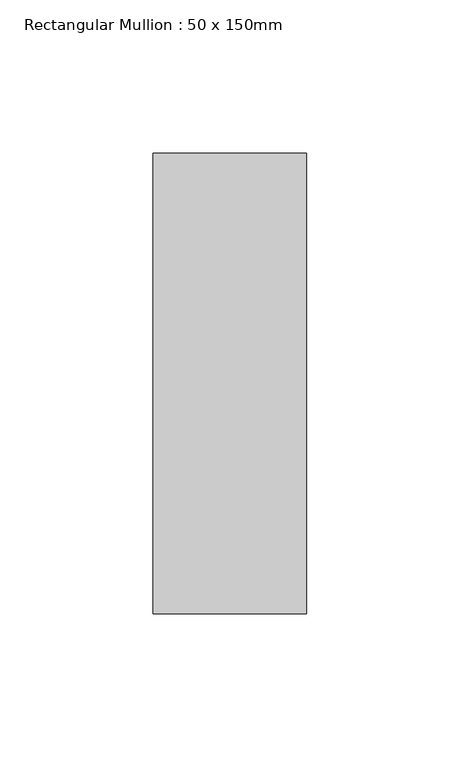
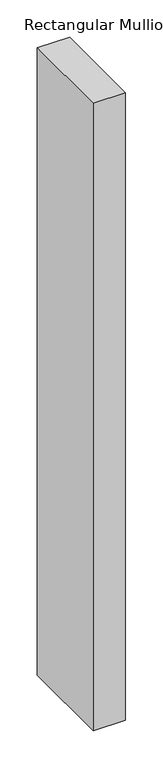
"""IFC4 building model written with IfcOpenShell, lengths in millimetres: member geometry, Rectangular Mullion : 50 x 150mm."""

from ifc_helpers import new_model, si_unit, frame, origin, place, context, project, spatial, polyline, outline, extrude, source, transform, mapped, element, save


def rectangular_mullion_50_x_150mm_b402127a(model_context):
    return source(origin(), model_context, "Body", "SweptSolid", [
        extrude(outline(polyline([(25.0, 75.0), (25.0, -75.0), (-25.0, -75.0), (-25.0, 75.0), (25.0, 75.0)])), frame((0.0, 0.0, -1027.5595785), z_axis=(0.0, 0.0, 1.0), x_axis=(1.0, 0.0, 0.0)), (0.0, 0.0, 1.0), 1027.5595785),
    ])


if __name__ == "__main__":
    model = new_model("IFC4")
    model_context = context("Model", 3, world=origin())
    ifc_project = project(units=[si_unit("LENGTHUNIT", "METRE", prefix="MILLI")], contexts=[model_context])
    site = spatial("IfcSite", under=ifc_project)
    building = spatial("IfcBuilding", under=site)
    placement = place(None, origin())
    rectangular_mullion_50_x_150mm_shape = rectangular_mullion_50_x_150mm_b402127a(model_context)
    element("IfcMember", 1, ObjectType="Rectangular Mullion : 50 x 150mm", at=placement, inside=building, context=model_context, shape_type="MappedRepresentation", body=[
        mapped(rectangular_mullion_50_x_150mm_shape, transform((0.0, 0.0, 0.0), x_axis=(1.0, 0.0, 0.0), y_axis=(0.0, 1.0, 0.0), z_axis=(0.0, 0.0, 1.0))),
    ])
    save(model, "model.ifc")

# Revit data of these elements
# Type "Rectangular Mullion : 50 x 150mm"
#   built-in parameter 1007304 = 0.492126 (stored number, unit not read)
#   built-in parameter 1007301 = 0.082021 (stored number, unit not read)
#   built-in parameter 1007300 = 0.082021 (stored number, unit not read)
# Element 1 (IfcMember, "Rectangular Mullion : 50 x 150mm")
#   Materials on its faces: "Aluminium"
# Materials
#   "Aluminium": class "Metal", colour RGB 247 247 247, transparency 0, Description = "Aluminium 6061", Cost = 0
